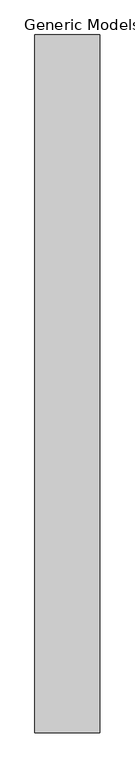
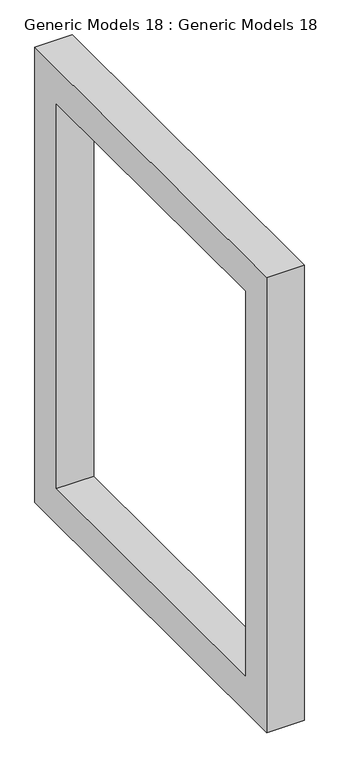
"""IFC4 building model written with IfcOpenShell, lengths in millimetres: proxy geometry, Generic Models 18 : Generic Models 18."""

from ifc_helpers import new_model, si_unit, frame, origin, place, context, project, spatial, polyline, outline, extrude, source, transform, mapped, element, save


def generic_models_18_generic_models_18_24b474a2(model_context):
    return source(origin(), model_context, "Body", "SweptSolid", [
        extrude(outline(polyline([(2275.0405883, 6000.75), (3913.3405883, 6000.75), (3913.3405883, 4035.4676291), (2275.0405883, 4035.4676291), (2275.0405883, 6000.75)]), holes=[polyline([(2427.4405883, 5848.35), (2427.4405883, 4187.8676291), (3760.9405883, 4187.8676291), (3760.9405883, 5848.35), (2427.4405883, 5848.35)])]), frame((-12202.0586008, 0.0, 0.0), z_axis=(1.0, 0.0, 0.0), x_axis=(0.0, 1.0, 0.0)), (0.0, 0.0, 1.0), 152.4),
    ])


if __name__ == "__main__":
    model = new_model("IFC4")
    model_context = context("Model", 3, world=origin())
    ifc_project = project(units=[si_unit("LENGTHUNIT", "METRE", prefix="MILLI")], contexts=[model_context])
    site = spatial("IfcSite", under=ifc_project)
    building = spatial("IfcBuilding", under=site)
    placement = place(None, origin())
    generic_models_18_generic_models_18_shape = generic_models_18_generic_models_18_24b474a2(model_context)
    element("IfcBuildingElementProxy", 1, Name="Generic Models 18 : Generic Models 18", ObjectType="Generic Models 18 : Generic Models 18", at=placement, inside=building, context=model_context, shape_type="MappedRepresentation", body=[
        mapped(generic_models_18_generic_models_18_shape, transform((0.0, 0.0, 0.0), x_axis=(1.0, 0.0, 0.0), y_axis=(0.0, 1.0, 0.0), z_axis=(0.0, 0.0, 1.0))),
    ])
    save(model, "model.ifc")

# Revit data of these elements
# Element 1 (IfcBuildingElementProxy, "Generic Models 18 : Generic Models 18")
#   Materials on its faces: "feature frame"
# Materials
#   "feature frame": class "Generic", colour RGB 120 120 120, transparency 0, Cost = 0
